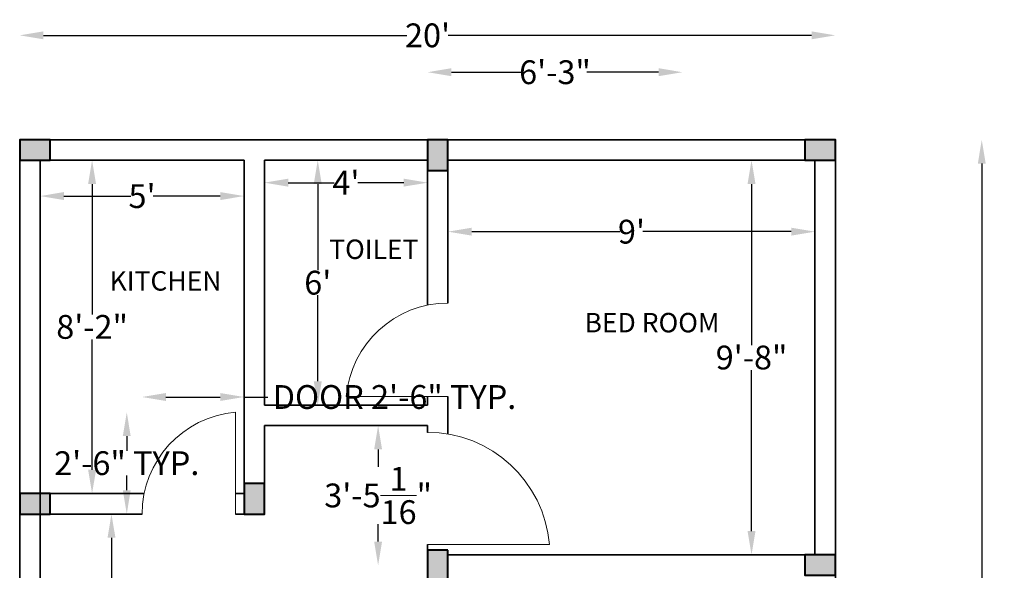
# Model space of a CAD drawing. Units: inches. Extents: x 2773 to 3100, y 2330 to 2750.
# Tile 2 of 2: x 2804 to 3093, y 2588 to 2750. Entities that reach past the tile are written whole.
import ezdxf

# ---------------------------------------------------------------- set-up
doc = ezdxf.new("R2010")
doc.units = ezdxf.units.IN
for name, color, linetype, lineweight in [('A-ANNO-DIMS', 2, 'Continuous', 18), ('A-AREA-IDEN', 7, 'Continuous', 18), ('A-COLS', 7, 'Continuous', 40), ('A-DOOR', 4, 'Continuous', 18), ('A-WALL', 7, 'Continuous', 35)]:
    doc.layers.add(name, color=color, linetype=linetype, lineweight=lineweight)
doc.styles.get("Standard").update_dxf_attribs({"font": 'arial.ttf'})
doc.dimstyles.get("Standard").update_dxf_attribs({"dimtxt": 7, "dimasz": 7, "dimexe": 0.18, "dimexo": 0.0625, "dimgap": 0.09, "dimtad": 0, "dimtih": 1, "dimtoh": 1, "dimdec": 4, "dimzin": 0, "dimdsep": 46, "dimlunit": 4, "dimtxsty": 'Standard', "dimcen": 0.09, "dimse1": 1, "dimse2": 1, "dimadec": 0, "dimazin": 0, "dimtfac": 1, "dimtdec": 4, "dimtofl": 0, "dimtmove": 0, "dimatfit": 3, "dimfxl": 1, "dimtolj": 1, "dimtzin": 0, "dimarcsym": 0})

# ---------------------------------------------------------------- blocks, each defined once
blk = doc.blocks.new('*D1')
at = {"layer": 'A-ANNO-DIMS', "color": 0, "lineweight": -2, "transparency": 16777216}
for p, q in [((2824.93, 2701.68), (2824.93, 2663.34)), ((2824.93, 2617.68), (2824.93, 2656.01))]:
    blk.add_line(p, q, dxfattribs=at)
at = {"layer": 'A-ANNO-DIMS', "color": 0, "transparency": 16777216}
for points in [[(2823.76, 2701.68), (2826.1, 2701.68), (2824.93, 2708.68)], [(2823.76, 2617.68), (2826.1, 2617.68), (2824.93, 2610.68)]]:
    blk.add_solid(points, dxfattribs=at)
at = {"layer": 'Defpoints', "color": 0, "transparency": 16777216}
for p in [(2809.63, 2708.68), (2809.63, 2610.68), (2824.93, 2610.68)]:
    blk.add_point(p, dxfattribs=at)
at = {"layer": 'A-ANNO-DIMS', "color": 0, "transparency": 16777216, "insert": (2824.93, 2659.68), "char_height": 7, "attachment_point": 5}
blk.add_mtext('\\A1;8\'-2"', dxfattribs=at)
blk = doc.blocks.new('*D2')
at = {"layer": 'A-ANNO-DIMS', "color": 0, "lineweight": -2, "transparency": 16777216}
for p, q in [((2816.63, 2698.14), (2836.32, 2698.14)), ((2862.63, 2698.14), (2842.94, 2698.14))]:
    blk.add_line(p, q, dxfattribs=at)
at = {"layer": 'A-ANNO-DIMS', "color": 0, "transparency": 16777216}
for points in [[(2816.63, 2699.31), (2816.63, 2696.97), (2809.63, 2698.14)], [(2862.63, 2699.31), (2862.63, 2696.97), (2869.63, 2698.14)]]:
    blk.add_solid(points, dxfattribs=at)
at = {"layer": 'Defpoints', "color": 0, "transparency": 16777216}
for p in [(2809.63, 2702.7), (2869.63, 2702.7), (2869.63, 2698.14)]:
    blk.add_point(p, dxfattribs=at)
at = {"layer": 'A-ANNO-DIMS', "color": 0, "transparency": 16777216, "insert": (2839.63, 2698.14), "char_height": 7, "attachment_point": 5}
blk.add_mtext("\\A1;5'", dxfattribs=at)
blk = doc.blocks.new('*D3')
at = {"layer": 'A-ANNO-DIMS', "color": 0, "lineweight": -2, "transparency": 16777216}
for p, q in [((2882.63, 2702.08), (2896.18, 2702.08)), ((2916.63, 2702.08), (2903.08, 2702.08))]:
    blk.add_line(p, q, dxfattribs=at)
at = {"layer": 'A-ANNO-DIMS', "color": 0, "transparency": 16777216}
for points in [[(2882.63, 2703.25), (2882.63, 2700.92), (2875.63, 2702.08)], [(2916.63, 2703.25), (2916.63, 2700.92), (2923.63, 2702.08)]]:
    blk.add_solid(points, dxfattribs=at)
at = {"layer": 'Defpoints', "color": 0, "transparency": 16777216}
for p in [(2875.63, 2702.64), (2923.63, 2702.64), (2923.63, 2702.08)]:
    blk.add_point(p, dxfattribs=at)
at = {"layer": 'A-ANNO-DIMS', "color": 0, "transparency": 16777216, "insert": (2899.63, 2702.08), "char_height": 7, "attachment_point": 5}
blk.add_mtext("\\A1;4'", dxfattribs=at)
blk = doc.blocks.new('*D4')
at = {"layer": 'A-ANNO-DIMS', "color": 0, "lineweight": -2, "transparency": 16777216}
for p, q in [((2891.33, 2701.68), (2891.33, 2676.34)), ((2891.33, 2643.68), (2891.33, 2669.01))]:
    blk.add_line(p, q, dxfattribs=at)
at = {"layer": 'A-ANNO-DIMS', "color": 0, "transparency": 16777216}
for points in [[(2890.16, 2701.68), (2892.5, 2701.68), (2891.33, 2708.68)], [(2890.16, 2643.68), (2892.5, 2643.68), (2891.33, 2636.68)]]:
    blk.add_solid(points, dxfattribs=at)
at = {"layer": 'Defpoints', "color": 0, "transparency": 16777216}
for p in [(2884.28, 2708.68), (2884.28, 2636.68), (2891.33, 2636.68)]:
    blk.add_point(p, dxfattribs=at)
at = {"layer": 'A-ANNO-DIMS', "color": 0, "transparency": 16777216, "insert": (2891.33, 2672.68), "char_height": 7, "attachment_point": 5}
blk.add_mtext("\\A1;6'", dxfattribs=at)
blk = doc.blocks.new('*D5')
at = {"layer": 'A-ANNO-DIMS', "color": 0, "lineweight": -2, "transparency": 16777216}
for p, q in [((3018.96, 2701.68), (3018.96, 2654.34)), ((3018.96, 2599.68), (3018.96, 2647.01))]:
    blk.add_line(p, q, dxfattribs=at)
at = {"layer": 'A-ANNO-DIMS', "color": 0, "transparency": 16777216}
for points in [[(3017.79, 2701.68), (3020.12, 2701.68), (3018.96, 2708.68)], [(3017.79, 2599.68), (3020.12, 2599.68), (3018.96, 2592.68)]]:
    blk.add_solid(points, dxfattribs=at)
at = {"layer": 'Defpoints', "color": 0, "transparency": 16777216}
for p in [(3000.78, 2708.68), (3000.78, 2592.68), (3018.96, 2592.68)]:
    blk.add_point(p, dxfattribs=at)
at = {"layer": 'A-ANNO-DIMS', "color": 0, "transparency": 16777216, "insert": (3018.96, 2650.68), "char_height": 7, "attachment_point": 5}
blk.add_mtext('\\A1;9\'-8"', dxfattribs=at)
blk = doc.blocks.new('*D6')
at = {"layer": 'A-ANNO-DIMS', "color": 0, "lineweight": -2, "transparency": 16777216}
for p, q in [((2936.63, 2687.68), (2980.32, 2687.68)), ((3030.63, 2687.68), (2986.94, 2687.68))]:
    blk.add_line(p, q, dxfattribs=at)
at = {"layer": 'A-ANNO-DIMS', "color": 0, "transparency": 16777216}
for points in [[(2936.63, 2688.84), (2936.63, 2686.51), (2929.63, 2687.68)], [(3030.63, 2688.84), (3030.63, 2686.51), (3037.63, 2687.68)]]:
    blk.add_solid(points, dxfattribs=at)
at = {"layer": 'Defpoints', "color": 0, "transparency": 16777216}
for p in [(2929.63, 2687.68), (3037.63, 2687.68), (3037.63, 2687.68)]:
    blk.add_point(p, dxfattribs=at)
at = {"layer": 'A-ANNO-DIMS', "color": 0, "transparency": 16777216, "insert": (2983.63, 2687.68), "char_height": 7, "attachment_point": 5}
blk.add_mtext("\\A1;9'", dxfattribs=at)
blk = doc.blocks.new('*D11')
at = {"layer": 'A-ANNO-DIMS', "color": 0, "lineweight": -2, "transparency": 16777216}
for p, q in [((2909.09, 2623.68), (2909.09, 2618.54)), ((2909.09, 2596.59), (2909.09, 2601.72))]:
    blk.add_line(p, q, dxfattribs=at)
at = {"layer": 'A-ANNO-DIMS', "color": 0, "transparency": 16777216}
for points in [[(2907.92, 2623.68), (2910.25, 2623.68), (2909.09, 2630.68)], [(2907.92, 2596.59), (2910.25, 2596.59), (2909.09, 2589.59)]]:
    blk.add_solid(points, dxfattribs=at)
at = {"layer": 'Defpoints', "color": 0, "transparency": 16777216}
for p in [(2911.25, 2630.68), (2909.09, 2589.59), (2911.25, 2589.59)]:
    blk.add_point(p, dxfattribs=at)
at = {"layer": 'A-ANNO-DIMS', "color": 0, "transparency": 16777216, "insert": (2909.09, 2610.13), "char_height": 7, "attachment_point": 5}
blk.add_mtext('\\A1;3\'-5{\\H1x;\\S1/16;}"', dxfattribs=at)
blk = doc.blocks.new('*D12')
at = {"layer": 'A-ANNO-DIMS', "color": 0, "lineweight": -2, "transparency": 16777216}
for p, q in [((2830.63, 2597.68), (2830.63, 2555.84)), ((2830.63, 2506.68), (2830.63, 2548.51))]:
    blk.add_line(p, q, dxfattribs=at)
at = {"layer": 'A-ANNO-DIMS', "color": 0, "transparency": 16777216}
for points in [[(2829.47, 2597.68), (2831.8, 2597.68), (2830.63, 2604.68)], [(2829.47, 2506.68), (2831.8, 2506.68), (2830.63, 2499.68)]]:
    blk.add_solid(points, dxfattribs=at)
at = {"layer": 'Defpoints', "color": 0, "transparency": 16777216}
for p in [(2829.2, 2604.68), (2829.2, 2499.68), (2830.63, 2499.68)]:
    blk.add_point(p, dxfattribs=at)
at = {"layer": 'A-ANNO-DIMS', "color": 0, "transparency": 16777216, "insert": (2830.63, 2552.18), "char_height": 7, "attachment_point": 5}
blk.add_mtext('\\A1;8\'-9"', dxfattribs=at)
blk = doc.blocks.new('*D15')
at = {"layer": 'A-ANNO-DIMS', "color": 0, "lineweight": -2, "transparency": 16777216}
for p, q in [((2810.63, 2745.39), (2917.54, 2745.39)), ((3036.63, 2745.39), (2929.72, 2745.39))]:
    blk.add_line(p, q, dxfattribs=at)
at = {"layer": 'A-ANNO-DIMS', "color": 0, "transparency": 16777216}
for points in [[(2810.63, 2746.56), (2810.63, 2744.23), (2803.63, 2745.39)], [(3036.63, 2746.56), (3036.63, 2744.23), (3043.63, 2745.39)]]:
    blk.add_solid(points, dxfattribs=at)
at = {"layer": 'Defpoints', "color": 0, "transparency": 16777216}
for p in [(3043.63, 2745.39), (2803.63, 2714.68), (3043.63, 2714.68)]:
    blk.add_point(p, dxfattribs=at)
at = {"layer": 'A-ANNO-DIMS', "color": 0, "transparency": 16777216, "insert": (2923.63, 2745.39), "char_height": 7, "attachment_point": 5}
blk.add_mtext("\\A1;20'", dxfattribs=at)
blk = doc.blocks.new('*D16')
at = {"layer": 'A-ANNO-DIMS', "color": 0, "lineweight": -2, "transparency": 16777216}
for p, q in [((3086.7, 2707.68), (3086.7, 2538.34)), ((3086.7, 2361.68), (3086.7, 2531.01))]:
    blk.add_line(p, q, dxfattribs=at)
at = {"layer": 'A-ANNO-DIMS', "color": 0, "transparency": 16777216}
for points in [[(3085.54, 2707.68), (3087.87, 2707.68), (3086.7, 2714.68)], [(3085.54, 2361.68), (3087.87, 2361.68), (3086.7, 2354.68)]]:
    blk.add_solid(points, dxfattribs=at)
at = {"layer": 'Defpoints', "color": 0, "transparency": 16777216}
for p in [(3043.63, 2714.68), (3043.63, 2354.68), (3086.7, 2354.68)]:
    blk.add_point(p, dxfattribs=at)
at = {"layer": 'A-ANNO-DIMS', "color": 0, "transparency": 16777216, "insert": (3086.7, 2534.68), "char_height": 7, "attachment_point": 5}
blk.add_mtext("\\A1;30'", dxfattribs=at)
blk = doc.blocks.new('COL-9X6')
h = blk.add_hatch(color=256)
h.dxf.hatch_style = 1
h.paths.add_polyline_path([(0, 6), (0, 0), (9, 0), (9, 6)])
blk.add_lwpolyline([(9, 0), (9, 6), (0, 6), (0, 0)], close=True)
blk = doc.blocks.new('COL-6X9')
h = blk.add_hatch(color=256)
h.dxf.hatch_style = 1
h.paths.add_polyline_path([(6, 9), (0, 9), (0, 0), (6, 0)])
blk.add_lwpolyline([(6, 9), (0, 9), (0, 0), (6, 0)], close=True)
blk = doc.blocks.new('DOOR-SWING-30')
for p, q in [((-2.5, 29.9), (-2.5, 0)), ((0, 0), (-2.5, 0)), ((-2.5, 0), (0, 0))]:
    blk.add_line(p, q)
blk.add_arc((0, 0), 30, 94.7802, 180)
blk = doc.blocks.new('DOOR-SWING-36')
for p, q in [((-3, 35.87), (-3, 0)), ((0, 6), (0, 36)), ((0, 36), (0, 6))]:
    blk.add_line(p, q)
blk.add_arc((0, 0), 36, 94.7802, 180)
blk = doc.blocks.new('*D27')
at = {"layer": 'A-ANNO-DIMS', "color": 0, "lineweight": -2, "transparency": 16777216}
for p, q in [((2846.63, 2639.07), (2862.63, 2639.07)), ((2869.63, 2639.07), (2876.63, 2639.07))]:
    blk.add_line(p, q, dxfattribs=at)
at = {"layer": 'A-ANNO-DIMS', "color": 0, "transparency": 16777216}
for points in [[(2846.63, 2640.24), (2846.63, 2637.91), (2839.63, 2639.07)], [(2862.63, 2640.24), (2862.63, 2637.91), (2869.63, 2639.07)]]:
    blk.add_solid(points, dxfattribs=at)
at = {"layer": 'Defpoints', "color": 0, "transparency": 16777216}
for p in [(2869.63, 2639.07), (2839.63, 2634.57), (2869.63, 2634.57)]:
    blk.add_point(p, dxfattribs=at)
at = {"layer": 'A-ANNO-DIMS', "color": 0, "transparency": 16777216, "insert": (2913.9, 2639.07), "char_height": 7, "attachment_point": 5}
blk.add_mtext('\\A1;DOOR 2\'-6" TYP.', dxfattribs=at)
blk = doc.blocks.new('*D28')
at = {"layer": 'A-ANNO-DIMS', "color": 0, "lineweight": -2, "transparency": 16777216}
for p, q in [((2835.13, 2627.57), (2835.13, 2623.29)), ((2835.13, 2611.68), (2835.13, 2615.96))]:
    blk.add_line(p, q, dxfattribs=at)
at = {"layer": 'A-ANNO-DIMS', "color": 0, "transparency": 16777216}
for points in [[(2833.96, 2627.57), (2836.29, 2627.57), (2835.13, 2634.57)], [(2833.96, 2611.68), (2836.29, 2611.68), (2835.13, 2604.68)]]:
    blk.add_solid(points, dxfattribs=at)
at = {"layer": 'Defpoints', "color": 0, "transparency": 16777216}
for p in [(2835.13, 2634.57), (2839.63, 2634.57), (2839.63, 2604.68)]:
    blk.add_point(p, dxfattribs=at)
at = {"layer": 'A-ANNO-DIMS', "color": 0, "transparency": 16777216, "insert": (2835.13, 2619.62), "char_height": 7, "attachment_point": 5}
blk.add_mtext('\\A1;2\'-6" TYP.', dxfattribs=at)
blk = doc.blocks.new('*D38')
at = {"layer": 'A-ANNO-DIMS', "color": 0, "lineweight": -2, "transparency": 16777216}
for p, q in [((2930.63, 2734.55), (2951.71, 2734.55)), ((2991.63, 2734.55), (2970.54, 2734.55))]:
    blk.add_line(p, q, dxfattribs=at)
at = {"layer": 'A-ANNO-DIMS', "color": 0, "transparency": 16777216}
for points in [[(2930.63, 2735.72), (2930.63, 2733.39), (2923.63, 2734.55)], [(2991.63, 2735.72), (2991.63, 2733.39), (2998.63, 2734.55)]]:
    blk.add_solid(points, dxfattribs=at)
at = {"layer": 'Defpoints', "color": 0, "transparency": 16777216}
for p in [(2998.63, 2734.55), (2923.63, 2432.68), (2998.63, 2432.68)]:
    blk.add_point(p, dxfattribs=at)
at = {"layer": 'A-ANNO-DIMS', "color": 0, "transparency": 16777216, "insert": (2961.13, 2734.55), "char_height": 7, "attachment_point": 5}
blk.add_mtext('\\A1;6\'-3"', dxfattribs=at)

msp = doc.modelspace()

# ---------------------------------------------------------------- linework, layer by layer
at = {"layer": 'A-DOOR'}
for p, q in [((2923.62737, 2636.67688), (2899.62737, 2636.67688)), ((2899.62737, 2636.67688), (2923.62737, 2636.67688)), ((2869.62737, 2610.67688), (2869.62737, 2634.67688)), ((2869.62737, 2634.67688), (2869.62737, 2610.67688)), ((2923.62737, 2591.08543), (2923.62737, 2594.08543)), ((2923.62737, 2594.08543), (2923.62737, 2591.08543))]:
    msp.add_line(p, q, dxfattribs=at)
at = {"layer": 'A-WALL'}
for p, q in [((2803.62737, 2714.67688), (2803.62737, 2354.67688)), ((3043.62737, 2714.67688), (2803.62737, 2714.67688)), ((3043.62737, 2354.67688), (3043.62737, 2714.67688)), ((2809.62737, 2708.67688), (2809.62737, 2499.67688)), ((2869.62737, 2708.67688), (2809.62737, 2708.67688)), ((2869.62737, 2708.67688), (2869.62737, 2610.67688)), ((2875.62737, 2708.67688), (2875.62737, 2636.67688)), ((2923.62737, 2708.67688), (2875.62737, 2708.67688)), ((2923.62737, 2708.67688), (2923.62737, 2666.07076)), ((2929.62737, 2708.67688), (2929.62737, 2666.67688)), ((3037.62737, 2708.67688), (2929.62737, 2708.67688)), ((3037.62737, 2592.67688), (3037.62737, 2708.67688)), ((2923.62737, 2636.67688), (2875.62737, 2636.67688)), ((2923.62737, 2639.17688), (2923.62737, 2636.67688)), ((2929.62737, 2639.17688), (2929.62737, 2628.17336)), ((2923.62737, 2630.67688), (2875.62737, 2630.67688)), ((2875.62737, 2630.67688), (2875.62737, 2604.67688)), ((2923.62737, 2630.67688), (2923.62737, 2628.67688)), ((2840.23349, 2610.67688), (2809.62737, 2610.67688)), ((2869.62737, 2610.67688), (2867.12737, 2610.67688)), ((2839.62737, 2604.67688), (2809.62737, 2604.67688)), ((2875.62737, 2604.67688), (2867.12737, 2604.67688)), ((2923.62737, 2595.67688), (2923.62737, 2583.67688)), ((2929.62737, 2594.08543), (2929.62737, 2591.08543)), ((2929.62737, 2592.67688), (3037.62737, 2592.67688))]:
    msp.add_line(p, q, dxfattribs=at)

# ---------------------------------------------------------------- block references
at = {"layer": 'A-COLS'}
for name, p in [('COL-9X6', (2803.62737, 2708.67688)), ('COL-6X9', (2923.62737, 2705.67688)), ('COL-9X6', (3034.62737, 2708.67688)), ('COL-6X9', (2869.62737, 2604.67688)), ('COL-9X6', (2803.62737, 2604.67688)), ('COL-9X6', (3034.62737, 2586.67688))]:
    msp.add_blockref(name, p, dxfattribs=at)
at = {"layer": 'A-COLS', "rotation": 89.99999999999864}
msp.add_blockref('COL-9X6', (2929.62737, 2585.08543), dxfattribs=at)
at = {"layer": 'A-DOOR', "extrusion": (0, 0, -1), "zscale": -1, "rotation": 269.9999999999981}
msp.add_blockref('DOOR-SWING-30', (-2929.62737, 2636.67688), dxfattribs=at)
at = {"layer": 'A-DOOR'}
msp.add_blockref('DOOR-SWING-30', (2869.62737, 2604.67688), dxfattribs=at)
at = {"layer": 'A-DOOR', "rotation": 270.000000000001}
msp.add_blockref('DOOR-SWING-36', (2923.62737, 2592.67688), dxfattribs=at)

# ---------------------------------------------------------------- texts
at = {"layer": 'A-AREA-IDEN', "char_height": 5.720006, "attachment_point": 1}
for s, insert in [('TOILET', (2894.70132, 2685.36657)), ('KITCHEN', (2830.09824, 2676.06333)), ('BED ROOM', (2969.8105, 2663.78891))]:
    msp.add_mtext_dynamic_manual_height_columns(s, width=353.6359827, gutter_width=28.60003, heights=[0], dxfattribs=dict(at, insert=insert))

# ---------------------------------------------------------------- dimensions: what is measured, and where the dimension line sits
at = {"layer": 'A-ANNO-DIMS'}
for base, p1, p2, override, picture, middle in [((3043.62737, 2745.39262), (2803.62737, 2714.67688), (3043.62737, 2714.67688), {"dimclrd": 0, "dimclre": 0, "dimclrt": 0}, '*D15', (2923.62737, 2745.39262)), ((2998.62737, 2734.55188), (2923.62737, 2432.67688), (2998.62737, 2432.67688), {"dimdec": 1, "dimlfac": 1, "dimrnd": 0, "dimzin": 1, "dimdsep": 46, "dimlunit": 4, "dimfrac": 2}, '*D38', (2961.12737, 2734.55188)), ((2923.62737, 2702.0829), (2875.62737, 2702.63564), (2923.62737, 2702.63564), {"dimclrd": 0, "dimclre": 0, "dimclrt": 0}, '*D3', (2899.62737, 2702.0829)), ((2869.62737, 2698.1403), (2809.62737, 2702.70192), (2869.62737, 2702.70192), {"dimclrd": 0, "dimclre": 0, "dimclrt": 0}, '*D2', (2839.62737, 2698.1403)), ((3037.62737, 2687.67688), (2929.62737, 2687.67688), (3037.62737, 2687.67688), {"dimclrd": 0, "dimclre": 0, "dimclrt": 0}, '*D6', (2983.62737, 2687.67688))]:
    dim = msp.add_linear_dim(base=base, p1=p1, p2=p2, dimstyle='Standard', override=override, dxfattribs=at)
    dim.commit()
    dim.dimension.update_dxf_attribs({"geometry": picture, "text_midpoint": middle})
for base, p1, p2, override, picture, middle in [((3086.70499, 2354.67688), (3043.62737, 2714.67688), (3043.62737, 2354.67688), {"dimclrd": 0, "dimclre": 0, "dimclrt": 0}, '*D16', (3086.70499, 2534.67688)), ((2824.93043, 2610.67688), (2809.62737, 2708.67688), (2809.62737, 2610.67688), {"dimasz": 7, "dimclrd": 0, "dimclre": 0, "dimclrt": 0}, '*D1', (2824.93043, 2659.67688)), ((2891.33158, 2636.67688), (2884.27702, 2708.67688), (2884.27702, 2636.67688), {"dimclrd": 0, "dimclre": 0, "dimclrt": 0}, '*D4', (2891.33158, 2672.67688)), ((3018.95771, 2592.67688), (3000.78114, 2708.67688), (3000.78114, 2592.67688), {"dimclrd": 0, "dimclre": 0, "dimclrt": 0}, '*D5', (3018.95771, 2650.67688)), ((2909.086929, 2589.585434), (2911.253785, 2630.676883), (2911.253785, 2589.585434), {"dimclrd": 0, "dimclre": 0, "dimclrt": 0}, '*D11', (2909.086929, 2610.131158)), ((2830.63357, 2499.67688), (2829.20079, 2604.67688), (2829.20079, 2499.67688), {"dimclrd": 0, "dimclre": 0, "dimclrt": 0}, '*D12', (2830.63357, 2552.17688))]:
    dim = msp.add_linear_dim(base=base, p1=p1, p2=p2, angle=90, dimstyle='Standard', override=override, dxfattribs=at)
    dim.commit()
    dim.dimension.update_dxf_attribs({"geometry": picture, "text_midpoint": middle})
dim = msp.add_linear_dim(base=(2869.62737, 2639.07253), p1=(2839.62737, 2634.57253), p2=(2869.62737, 2634.57253), text='DOOR <> TYP.', dimstyle='Standard', override={"dimdec": 1, "dimlfac": 1, "dimrnd": 0, "dimzin": 1, "dimdsep": 46, "dimlunit": 4, "dimfrac": 2}, dxfattribs=at)
dim.commit()
dim.dimension.update_dxf_attribs({"geometry": '*D27', "text_midpoint": (2913.90427, 2639.07253)})
dim = msp.add_linear_dim(base=(2835.12737, 2634.57253), p1=(2839.62737, 2604.67688), p2=(2839.62737, 2634.57253), angle=90, text='<> TYP.', dimstyle='Standard', override={"dimdec": 1, "dimlfac": 1, "dimrnd": 0, "dimzin": 1, "dimdsep": 46, "dimlunit": 4, "dimfrac": 2}, dxfattribs=at)
dim.commit()
dim.dimension.update_dxf_attribs({"geometry": '*D28', "text_midpoint": (2835.12737, 2619.62471)})

doc.saveas('drawing.dxf')
